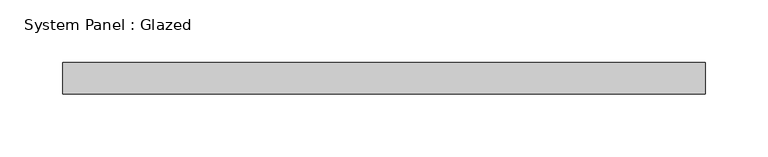
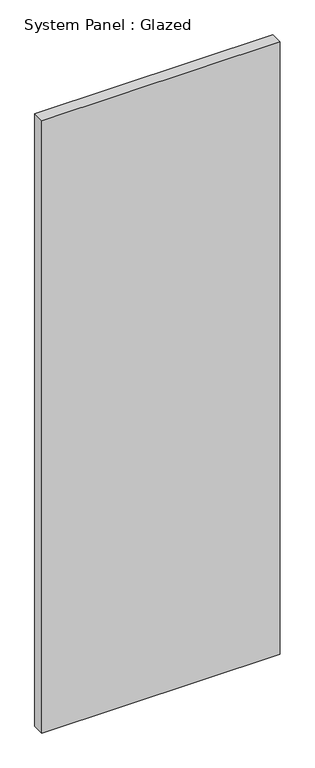
"""IFC4 building model written with IfcOpenShell, lengths in millimetres: plate geometry, System Panel : Glazed."""

from ifc_helpers import new_model, si_unit, origin, origin_with_axes, place, context, project, spatial, polyline, outline, extrude, source, transform, mapped, element, save


def system_panel_glazed_24803b90(model_context):
    return source(origin(), model_context, "Body", "SweptSolid", [
        extrude(outline(polyline([(257.175, 19.05), (-257.175, 19.05), (-257.175, 44.45), (257.175, 44.45), (257.175, 19.05)])), origin_with_axes(), (0.0, 0.0, 1.0), 1397.0),
    ])


if __name__ == "__main__":
    model = new_model("IFC4")
    model_context = context("Model", 3, world=origin())
    ifc_project = project(units=[si_unit("LENGTHUNIT", "METRE", prefix="MILLI")], contexts=[model_context])
    site = spatial("IfcSite", under=ifc_project)
    building = spatial("IfcBuilding", under=site)
    placement = place(None, origin())
    system_panel_glazed_shape = system_panel_glazed_24803b90(model_context)
    element("IfcPlate", 1, ObjectType="System Panel : Glazed", at=placement, inside=building, context=model_context, shape_type="MappedRepresentation", body=[
        mapped(system_panel_glazed_shape, transform((0.0, 0.0, 0.0), x_axis=(1.0, 0.0, 0.0), y_axis=(0.0, 1.0, 0.0), z_axis=(0.0, 0.0, 1.0))),
    ])
    save(model, "model.ifc")

# Revit data of these elements
# Type "System Panel : Glazed"
#   Construction Type Id = "GSP4R"
#   Analytic Construction = "1/8 in Pilkington single glazing"
#   Visual Light Transmittance = 0.9
#   Solar Heat Gain Coefficient = 0.86
#   Heat Transfer Coefficient (U) = 1.18115 BTU/(h·ft²·°F)
#   Define Thermal Properties by = 1
# Element 1 (IfcPlate, "System Panel : Glazed")
#   Materials on its faces: "Glass"
# Materials
#   "Glass": class "Glass", colour RGB 0 128 192, transparency 0.75, Description = "Soda Lime Glass", Cost = 0
